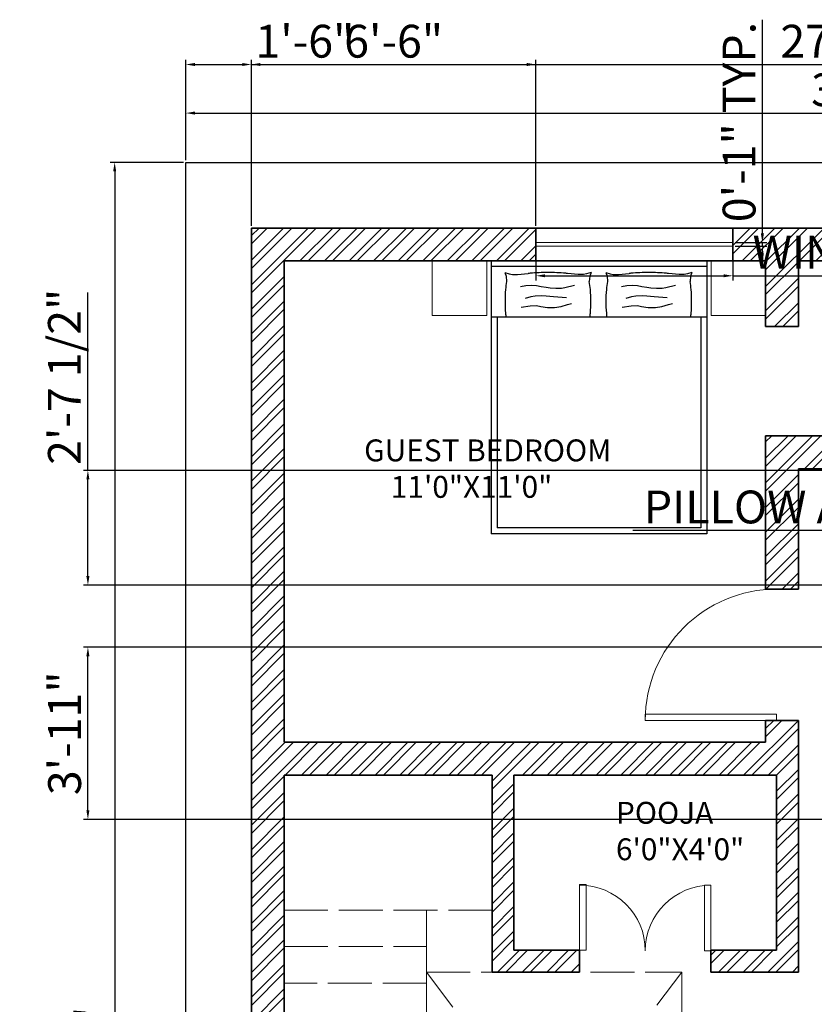
# Model space of a CAD drawing. Units: inches. Extents: x 638 to 1853, y 4393 to 5041.
# Tile 2 of 6: x 638 to 856, y 4693 to 4963. Entities that reach past the tile are written whole.
import ezdxf

# ---------------------------------------------------------------- set-up
doc = ezdxf.new("R2010")
doc.units = ezdxf.units.IN
doc.linetypes.add('ACAD_ISO02W100', pattern=[15, 12, -3])
for name, color, linetype, lineweight in [('A-ANNO-DIMS', 2, 'Continuous', 18), ('A-AREA-IDEN', 7, 'Continuous', 18), ('A-DOOR', 4, 'Continuous', 18), ('A-FLOR-STRS', 7, 'Continuous', 18), ('A-FLOR-STRS-HIDN', 7, 'ACAD_ISO02W100', 18), ('A-FURN', 26, 'Continuous', 13), ('A-GLAZ', 5, 'Continuous', 18), ('A-WALL', 7, 'Continuous', 35), ('A-WALL-PATT', 251, 'Continuous', 13), ('C-PROP', 7, 'Continuous', 25)]:
    doc.layers.add(name, color=color, linetype=linetype, lineweight=lineweight)
doc.layers.add('supurgelik', color=31, linetype='Continuous')
doc.layers.add('TASLAR', color=32, linetype='Continuous')
doc.styles.get("Standard").update_dxf_attribs({"font": 'arial.ttf'})
doc.dimstyles.new('ISO-25', dxfattribs={"dimtxt": 9, "dimasz": 2.5, "dimexe": 1.25, "dimexo": 0.625, "dimtad": 1, "dimdec": 1, "dimlunit": 3, "dimtxsty": 'Standard', "dimcen": 2.5, "dimadec": 0, "dimazin": 0, "dimtfac": 1, "dimtdec": 1, "dimtmove": 0, "dimatfit": 3, "dimfxl": 1, "dimarcsym": 0})

# ---------------------------------------------------------------- blocks, each defined once
blk = doc.blocks.new('*U4')
for p, q in [((0, 0), (0, -6)), ((36, 0), (36, -6))]:
    blk.add_line(p, q)
blk.add_lwpolyline([(0, 0), (0, 36), (1.75, 36), (1.75, 0)], close=True)
blk.add_arc((0, 0), 36, 0, 90)
blk = doc.blocks.new('hgjgh')
at = {"layer": 'supurgelik'}
for p, q in [((85993.81, -4751.89), (85843.81, -4751.89)), ((85853.26, -4756.05), (85856.29, -4757)), ((85853.26, -4756.05), (85854.18, -4758.49)), ((85854.18, -4758.49), (85854.49, -4762.19)), ((85856.29, -4757), (85858.52, -4757.5)), ((85858.52, -4757.5), (85862.12, -4757.37)), ((85862.12, -4757.37), (85869.57, -4756.72)), ((85904.4, -4757.37), (85896.95, -4756.72)), ((85908, -4757.5), (85904.4, -4757.37)), ((85910.23, -4757), (85908, -4757.5)), ((85913.26, -4756.05), (85910.23, -4757)), ((85912.34, -4758.49), (85912.03, -4762.19)), ((85913.26, -4756.05), (85912.34, -4758.49)), ((85923.48, -4756.05), (85926.51, -4757)), ((85923.48, -4756.05), (85924.4, -4758.49)), ((85924.4, -4758.49), (85924.71, -4762.19)), ((85926.51, -4757), (85928.74, -4757.5)), ((85928.74, -4757.5), (85932.34, -4757.37)), ((85932.34, -4757.37), (85939.79, -4756.72)), ((85974.62, -4757.37), (85967.17, -4756.72)), ((85978.22, -4757.5), (85974.62, -4757.37)), ((85980.45, -4757), (85978.22, -4757.5)), ((85983.48, -4756.05), (85980.45, -4757)), ((85982.56, -4758.49), (85982.25, -4762.19)), ((85983.48, -4756.05), (85982.56, -4758.49)), ((85864.23, -4765.86), (85867.95, -4764.99)), ((85867.95, -4764.99), (85871.91, -4764.87)), ((85871.91, -4764.87), (85875.39, -4765.12)), ((85875.39, -4765.12), (85878.49, -4765.74)), ((85895.1, -4766.36), (85901.8, -4764.87)), ((85934.44, -4765.86), (85938.16, -4764.99)), ((85938.16, -4764.99), (85942.13, -4764.87)), ((85942.13, -4764.87), (85945.6, -4765.12)), ((85945.6, -4765.12), (85948.7, -4765.74)), ((85965.32, -4766.36), (85972.02, -4764.87)), ((85878.86, -4772.3), (85874.27, -4772.55)), ((85878.49, -4765.74), (85881.96, -4766.23)), ((85881.96, -4772.55), (85878.86, -4772.3)), ((85881.96, -4766.23), (85884.81, -4766.61)), ((85884.81, -4766.61), (85888.65, -4766.85)), ((85888.65, -4766.85), (85892.62, -4766.85)), ((85892.62, -4766.85), (85895.1, -4766.36)), ((85949.08, -4772.3), (85944.49, -4772.55)), ((85948.7, -4765.74), (85952.18, -4766.23)), ((85952.18, -4772.55), (85949.08, -4772.3)), ((85952.18, -4766.23), (85955.03, -4766.61)), ((85955.03, -4766.61), (85958.87, -4766.85)), ((85958.87, -4766.85), (85962.84, -4766.85)), ((85962.84, -4766.85), (85965.32, -4766.36)), ((85871.29, -4773.05), (85867.33, -4774.04)), ((85870.92, -4779.28), (85875.39, -4779.03)), ((85874.27, -4772.55), (85871.29, -4773.05)), ((85875.39, -4779.03), (85878.24, -4779.65)), ((85887.04, -4773.05), (85881.96, -4772.55)), ((85890.14, -4773.3), (85887.04, -4773.05)), ((85896.09, -4773.67), (85890.14, -4773.3)), ((85892.37, -4779.65), (85896.96, -4778.41)), ((85896.96, -4778.41), (85899.69, -4777.54)), ((85941.51, -4773.05), (85937.54, -4774.04)), ((85941.14, -4779.28), (85945.6, -4779.03)), ((85944.49, -4772.55), (85941.51, -4773.05)), ((85945.6, -4779.03), (85948.46, -4779.65)), ((85957.26, -4773.05), (85952.18, -4772.55)), ((85960.36, -4773.3), (85957.26, -4773.05)), ((85966.31, -4773.67), (85960.36, -4773.3)), ((85962.59, -4779.65), (85967.18, -4778.41)), ((85967.18, -4778.41), (85969.91, -4777.54)), ((85864.72, -4780.15), (85870.92, -4779.28)), ((85878.24, -4779.65), (85882.95, -4780.4)), ((85882.95, -4780.4), (85887.91, -4780.4)), ((85887.91, -4780.4), (85892.37, -4779.65)), ((85934.94, -4780.15), (85941.14, -4779.28)), ((85948.46, -4779.65), (85953.17, -4780.4)), ((85953.17, -4780.4), (85958.13, -4780.4)), ((85958.13, -4780.4), (85962.59, -4779.65)), ((85993.81, -4787.2), (85843.81, -4787.2)), ((85847.81, -4787.2), (85847.81, -4933.89)), ((85989.81, -4787.2), (85989.81, -4933.89)), ((85989.81, -4933.89), (85847.81, -4933.89))]:
    blk.add_line(p, q, dxfattribs=at)
for centre, radius, start, end in [((85877.36, -4828.49), 72.19, 95.13619, 96.19323), ((85883.26, -4894.18), 138.14, 90, 95.13619), ((85883.26, -4894.18), 138.14, 84.86381, 90), ((85889.16, -4828.49), 72.19, 83.80677, 84.86381), ((85947.57, -4828.49), 72.19, 95.13619, 96.19323), ((85953.48, -4894.18), 138.14, 90, 95.13619), ((85953.48, -4894.18), 138.14, 84.86381, 90), ((85959.38, -4828.49), 72.19, 83.80677, 84.86381), ((85905.8, -4772.08), 52.26, 169.08956, 175.30047), ((85860.72, -4772.08), 52.26, 4.69953, 10.91044), ((85976.02, -4772.08), 52.26, 169.08956, 175.30047), ((85930.94, -4772.08), 52.26, 4.69953, 10.91044), ((85954.09, -4776.05), 100.71, 175.30047, 180), ((85812.43, -4776.05), 100.71, 0, 4.69953), ((86024.31, -4776.05), 100.71, 175.30047, 180), ((85882.65, -4776.05), 100.71, 0, 4.69953), ((85954.09, -4776.05), 100.71, 180, 184.69953), ((85812.43, -4776.05), 100.71, 355.30047, 0), ((86024.31, -4776.05), 100.71, 180, 184.69953), ((85882.65, -4776.05), 100.71, 355.30047, 0), ((85905.8, -4780.02), 52.26, 184.69953, 187.89725), ((85860.72, -4780.02), 52.26, 352.10275, 355.30047), ((85976.02, -4780.02), 52.26, 184.69953, 187.89725), ((85930.94, -4780.02), 52.26, 352.10275, 355.30047)]:
    blk.add_arc(centre, radius, start, end, dxfattribs=at)
at = {"layer": 'TASLAR'}
for p, q in [((85843.81, -4747.89), (85843.81, -4937.89)), ((85993.81, -4747.89), (85843.81, -4747.89)), ((85993.81, -4747.89), (85993.81, -4937.89)), ((85993.81, -4937.89), (85843.81, -4937.89))]:
    blk.add_line(p, q, dxfattribs=at)
blk = doc.blocks.new('*D16')
at = {"layer": 'A-ANNO-DIMS', "color": 0, "lineweight": -2, "transparency": 16777216}
for p, q in [((683.34, 4924.82), (683.34, 4938.95)), ((685.84, 4937.7), (1040.84, 4937.7)), ((1043.34, 4924.82), (1043.34, 4938.95))]:
    blk.add_line(p, q, dxfattribs=at)
at = {"layer": 'A-ANNO-DIMS', "color": 0, "transparency": 16777216}
for points in [[(685.84, 4938.12), (685.84, 4937.29), (683.34, 4937.7)], [(1040.84, 4938.12), (1040.84, 4937.29), (1043.34, 4937.7)]]:
    blk.add_solid(points, dxfattribs=at)
at = {"layer": 'Defpoints', "color": 0, "transparency": 16777216}
for p in [(1043.34, 4937.7), (683.34, 4924.19), (1043.34, 4924.19)]:
    blk.add_point(p, dxfattribs=at)
at = {"layer": 'A-ANNO-DIMS', "color": 0, "transparency": 16777216, "insert": (863.34, 4942.93), "char_height": 9, "attachment_point": 5}
blk.add_mtext("30'", dxfattribs=at)
blk = doc.blocks.new('*D17')
at = {"layer": 'A-ANNO-DIMS', "color": 0, "lineweight": -2, "transparency": 16777216}
for p, q in [((682.72, 4924.19), (662.61, 4924.19)), ((663.86, 4921.69), (663.86, 4446.69)), ((682.72, 4444.19), (662.61, 4444.19))]:
    blk.add_line(p, q, dxfattribs=at)
at = {"layer": 'A-ANNO-DIMS', "color": 0, "transparency": 16777216}
for points in [[(663.44, 4921.69), (664.28, 4921.69), (663.86, 4924.19)], [(663.44, 4446.69), (664.28, 4446.69), (663.86, 4444.19)]]:
    blk.add_solid(points, dxfattribs=at)
at = {"layer": 'Defpoints', "color": 0, "transparency": 16777216}
for p in [(683.34, 4924.19), (663.86, 4444.19), (683.34, 4444.19)]:
    blk.add_point(p, dxfattribs=at)
at = {"layer": 'A-ANNO-DIMS', "color": 0, "transparency": 16777216, "insert": (658.64, 4684.19), "char_height": 9, "attachment_point": 5, "rotation": 90}
blk.add_mtext("40'", dxfattribs=at)
blk = doc.blocks.new('BED-NIGHTSTAND-15')
blk.add_lwpolyline([(0, 14.98), (14.98, 14.98), (14.98, 0), (0, 0)], close=True)
blk = doc.blocks.new('WINDOW-GLAZING-54IN')
for p, q in [((0, 1), (54, 1)), ((0, 0), (54, 0))]:
    blk.add_line(p, q)
blk = doc.blocks.new('STAIR-WELL-OPENING')
for p, q in [((0, 93), (70, 0)), ((0, 0), (70, 93))]:
    blk.add_line(p, q)
blk.add_lwpolyline([(0, 93), (70, 93), (70, 0), (0, 0)], close=True)
blk = doc.blocks.new('*D44')
at = {"layer": 'A-ANNO-DIMS', "color": 0, "lineweight": -2, "transparency": 16777216}
for p, q in [((926.95, 4824.56), (926.95, 4822.01)), ((939.81, 4824.56), (939.81, 4822.01)), ((926.95, 4823.26), (805.91, 4823.26)), ((937.31, 4823.26), (929.45, 4823.26))]:
    blk.add_line(p, q, dxfattribs=at)
at = {"layer": 'A-ANNO-DIMS', "color": 0, "transparency": 16777216}
for points in [[(929.45, 4823.67), (929.45, 4822.84), (926.95, 4823.26)], [(937.31, 4823.67), (937.31, 4822.84), (939.81, 4823.26)]]:
    blk.add_solid(points, dxfattribs=at)
at = {"layer": 'Defpoints', "color": 0, "transparency": 16777216}
for p in [(926.95, 4825.19), (939.81, 4825.19), (926.95, 4823.26)]:
    blk.add_point(p, dxfattribs=at)
at = {"layer": 'A-ANNO-DIMS', "color": 0, "transparency": 16777216, "insert": (865.18, 4828.54), "char_height": 9, "attachment_point": 5}
blk.add_mtext('PILLOW A 1\'-1" TYP.', dxfattribs=at)
blk = doc.blocks.new('*D46')
at = {"layer": 'A-ANNO-DIMS', "color": 0, "lineweight": -2, "transparency": 16777216}
for p, q in [((779.34, 4900.57), (779.34, 4891.84)), ((833.34, 4900.57), (833.34, 4891.84)), ((781.84, 4893.09), (830.84, 4893.09)), ((833.34, 4893.09), (950.98, 4893.09))]:
    blk.add_line(p, q, dxfattribs=at)
at = {"layer": 'A-ANNO-DIMS', "color": 0, "transparency": 16777216}
for points in [[(781.84, 4893.51), (781.84, 4892.68), (779.34, 4893.09)], [(830.84, 4893.51), (830.84, 4892.68), (833.34, 4893.09)]]:
    blk.add_solid(points, dxfattribs=at)
at = {"layer": 'Defpoints', "color": 0, "transparency": 16777216}
for p in [(779.34, 4901.19), (833.34, 4901.19), (833.34, 4893.09)]:
    blk.add_point(p, dxfattribs=at)
at = {"layer": 'A-ANNO-DIMS', "color": 0, "transparency": 16777216, "insert": (893.41, 4898.38), "char_height": 9, "attachment_point": 5}
blk.add_mtext('WINDOW 4\'-6" TYP.', dxfattribs=at)
blk = doc.blocks.new('*D47')
at = {"layer": 'A-ANNO-DIMS', "color": 0, "lineweight": -2, "transparency": 16777216}
for p, q in [((841.44, 4904.69), (841.44, 4963.3)), ((833.97, 4902.19), (842.69, 4902.19)), ((833.97, 4901.19), (842.69, 4901.19)), ((841.44, 4901.19), (841.44, 4902.19)), ((841.44, 4898.69), (841.44, 4896.19))]:
    blk.add_line(p, q, dxfattribs=at)
at = {"layer": 'A-ANNO-DIMS', "color": 0, "transparency": 16777216}
for points in [[(841.02, 4904.69), (841.86, 4904.69), (841.44, 4902.19)], [(841.02, 4898.69), (841.86, 4898.69), (841.44, 4901.19)]]:
    blk.add_solid(points, dxfattribs=at)
at = {"layer": 'Defpoints', "color": 0, "transparency": 16777216}
for p in [(833.34, 4902.19), (833.34, 4901.19), (841.44, 4902.19)]:
    blk.add_point(p, dxfattribs=at)
at = {"layer": 'A-ANNO-DIMS', "color": 0, "transparency": 16777216, "insert": (836.22, 4935.25), "char_height": 9, "attachment_point": 5, "rotation": 90}
blk.add_mtext('0\'-1" TYP.', dxfattribs=at)
blk = doc.blocks.new('*D62')
at = {"layer": 'A-ANNO-DIMS', "color": 0, "lineweight": -2, "transparency": 16777216}
for p, q in [((786.73, 4678.11), (786.73, 4689.96)), ((861.6, 4678.11), (861.6, 4689.96)), ((789.23, 4688.71), (859.1, 4688.71)), ((861.6, 4688.71), (964.27, 4688.71))]:
    blk.add_line(p, q, dxfattribs=at)
at = {"layer": 'A-ANNO-DIMS', "color": 0, "transparency": 16777216}
for points in [[(789.23, 4689.13), (789.23, 4688.3), (786.73, 4688.71)], [(859.1, 4689.13), (859.1, 4688.3), (861.6, 4688.71)]]:
    blk.add_solid(points, dxfattribs=at)
at = {"layer": 'Defpoints', "color": 0, "transparency": 16777216}
for p in [(861.6, 4688.71), (786.73, 4677.48), (861.6, 4677.48)]:
    blk.add_point(p, dxfattribs=at)
at = {"layer": 'A-ANNO-DIMS', "color": 0, "transparency": 16777216, "insert": (914.18, 4694), "char_height": 9, "attachment_point": 5}
blk.add_mtext('DINING SET 6\'-3"', dxfattribs=at)
blk = doc.blocks.new('*D74')
at = {"layer": 'A-ANNO-DIMS', "color": 0, "lineweight": -2, "transparency": 16777216}
for p, q in [((701.34, 4906.82), (701.34, 4952.27)), ((703.84, 4951.02), (1022.84, 4951.02)), ((1025.34, 4906.82), (1025.34, 4952.27))]:
    blk.add_line(p, q, dxfattribs=at)
at = {"layer": 'A-ANNO-DIMS', "color": 0, "transparency": 16777216}
for points in [[(703.84, 4951.44), (703.84, 4950.6), (701.34, 4951.02)], [(1022.84, 4951.44), (1022.84, 4950.6), (1025.34, 4951.02)]]:
    blk.add_solid(points, dxfattribs=at)
at = {"layer": 'Defpoints', "color": 0, "transparency": 16777216}
for p in [(1025.34, 4951.02), (701.34, 4906.19), (1025.34, 4906.19)]:
    blk.add_point(p, dxfattribs=at)
at = {"layer": 'A-ANNO-DIMS', "color": 0, "transparency": 16777216, "insert": (863.34, 4956.24), "char_height": 9, "attachment_point": 5}
blk.add_mtext('27\'-0"', dxfattribs=at)
blk = doc.blocks.new('*D76')
at = {"layer": 'A-ANNO-DIMS', "color": 0, "lineweight": -2, "transparency": 16777216}
for p, q in [((683.34, 4924.82), (683.34, 4952.27)), ((685.84, 4951.02), (698.84, 4951.02)), ((701.34, 4906.82), (701.34, 4952.27)), ((701.34, 4951.02), (728.17, 4951.02))]:
    blk.add_line(p, q, dxfattribs=at)
at = {"layer": 'A-ANNO-DIMS', "color": 0, "transparency": 16777216}
for points in [[(685.84, 4951.44), (685.84, 4950.6), (683.34, 4951.02)], [(698.84, 4951.44), (698.84, 4950.6), (701.34, 4951.02)]]:
    blk.add_solid(points, dxfattribs=at)
at = {"layer": 'Defpoints', "color": 0, "transparency": 16777216}
for p in [(701.34, 4951.02), (683.34, 4924.19), (701.34, 4906.19)]:
    blk.add_point(p, dxfattribs=at)
at = {"layer": 'A-ANNO-DIMS', "color": 0, "transparency": 16777216, "insert": (716, 4956.24), "char_height": 9, "attachment_point": 5}
blk.add_mtext('1\'-6"', dxfattribs=at)
blk = doc.blocks.new('*D80')
at = {"layer": 'A-ANNO-DIMS', "color": 0, "lineweight": -2, "transparency": 16777216}
for p, q in [((701.34, 4906.82), (701.34, 4952.27)), ((703.84, 4951.02), (776.84, 4951.02)), ((779.34, 4906.82), (779.34, 4952.27))]:
    blk.add_line(p, q, dxfattribs=at)
at = {"layer": 'A-ANNO-DIMS', "color": 0, "transparency": 16777216}
for points in [[(703.84, 4951.44), (703.84, 4950.6), (701.34, 4951.02)], [(776.84, 4951.44), (776.84, 4950.6), (779.34, 4951.02)]]:
    blk.add_solid(points, dxfattribs=at)
at = {"layer": 'Defpoints', "color": 0, "transparency": 16777216}
for p in [(779.34, 4951.02), (701.34, 4906.19), (779.34, 4906.19)]:
    blk.add_point(p, dxfattribs=at)
at = {"layer": 'A-ANNO-DIMS', "color": 0, "transparency": 16777216, "insert": (740.34, 4956.24), "char_height": 9, "attachment_point": 5}
blk.add_mtext('6\'-6"', dxfattribs=at)
blk = doc.blocks.new('*D85')
at = {"layer": 'A-ANNO-DIMS', "color": 0, "lineweight": -2, "transparency": 16777216}
for p, q in [((939.25, 4791.29), (655.27, 4791.29)), ((656.52, 4746.54), (656.52, 4788.79)), ((939.25, 4744.04), (655.27, 4744.04))]:
    blk.add_line(p, q, dxfattribs=at)
at = {"layer": 'A-ANNO-DIMS', "color": 0, "transparency": 16777216}
for points in [[(656.1, 4788.79), (656.93, 4788.79), (656.52, 4791.29)], [(656.1, 4746.54), (656.93, 4746.54), (656.52, 4744.04)]]:
    blk.add_solid(points, dxfattribs=at)
at = {"layer": 'Defpoints', "color": 0, "transparency": 16777216}
for p in [(656.52, 4791.29), (939.87, 4791.29), (939.87, 4744.04)]:
    blk.add_point(p, dxfattribs=at)
at = {"layer": 'A-ANNO-DIMS', "color": 0, "transparency": 16777216, "insert": (651.29, 4767.66), "char_height": 9, "attachment_point": 5, "rotation": 90}
blk.add_mtext('3\'-11"', dxfattribs=at)
blk = doc.blocks.new('*D87')
at = {"layer": 'A-ANNO-DIMS', "color": 0, "lineweight": -2, "transparency": 16777216}
for p, q in [((656.52, 4839.74), (656.52, 4888.54)), ((892.19, 4839.74), (655.27, 4839.74)), ((656.52, 4810.75), (656.52, 4837.24)), ((892.19, 4808.25), (655.27, 4808.25))]:
    blk.add_line(p, q, dxfattribs=at)
at = {"layer": 'A-ANNO-DIMS', "color": 0, "transparency": 16777216}
for points in [[(656.1, 4837.24), (656.93, 4837.24), (656.52, 4839.74)], [(656.1, 4810.75), (656.93, 4810.75), (656.52, 4808.25)]]:
    blk.add_solid(points, dxfattribs=at)
at = {"layer": 'Defpoints', "color": 0, "transparency": 16777216}
for p in [(656.52, 4839.74), (892.82, 4839.74), (892.82, 4808.25)]:
    blk.add_point(p, dxfattribs=at)
at = {"layer": 'A-ANNO-DIMS', "color": 0, "transparency": 16777216, "insert": (651.24, 4865.39), "char_height": 9, "attachment_point": 5, "rotation": 90}
blk.add_mtext('2\'-7 1/2"', dxfattribs=at)

msp = doc.modelspace()

# ---------------------------------------------------------------- hatches: boundary and pattern name
at = {"layer": 'A-WALL-PATT', "transparency": 33554687}
h = msp.add_hatch(dxfattribs=at)
h.set_pattern_fill('ANSI32', color=256, scale=0.5)
h.paths.add_polyline_path([(779.34, 4906.19), (701.34, 4906.19), (701.34, 4531.19), (710.34, 4531.19), (710.34, 4561.19), (758.34, 4561.19), (758.34, 4528.19), (764.34, 4528.19), (767.34, 4528.19), (767.34, 4561.19), (821.34, 4561.19), (821.34, 4570.19), (710.34, 4570.19), (710.34, 4756.19), (767.34, 4756.19), (767.34, 4702.19), (791.34, 4702.19), (791.34, 4708.19), (773.34, 4708.19), (773.34, 4756.19), (845.34, 4756.19), (845.34, 4708.19), (827.35, 4708.19), (827.35, 4705.02), (827.34, 4702.19), (851.34, 4702.19), (851.34, 4771.19), (845.34, 4771.19), (842.34, 4771.19), (842.34, 4765.19), (710.34, 4765.19), (710.34, 4897.19), (779.34, 4897.19)])
h.paths.add_polyline_path([(1025.34, 4906.19), (833.34, 4906.19), (833.34, 4897.19), (842.34, 4897.19), (842.34, 4882.21), (842.34, 4879.19), (851.34, 4879.19), (851.34, 4897.19), (914.34, 4897.19), (914.34, 4879.19), (920.34, 4879.19), (920.34, 4897.19), (1016.34, 4897.19), (1016.34, 4885.19), (1025.34, 4885.19)])
h.paths.add_polyline_path([(851.34, 4840.19), (1016.34, 4840.19), (1016.34, 4780.19), (1025.34, 4780.19), (1025.34, 4861.19), (1016.34, 4861.19), (1016.34, 4849.19), (842.34, 4849.19), (842.34, 4807.19), (851.34, 4807.19)])
h.paths.add_polyline_path([(1025.34, 4708.19), (1016.34, 4708.19), (1016.34, 4694.92), (1016.34, 4648.19), (996.84, 4648.19), (996.84, 4639.19), (1025.34, 4639.19)])
h.paths.add_polyline_path([(972.84, 4648.19), (944.34, 4648.19), (944.34, 4561.19), (953.34, 4561.19), (953.34, 4639.19), (972.84, 4639.19)])
h.paths.add_polyline_path([(896.34, 4648.19), (887.34, 4648.19), (887.34, 4570.19), (863.34, 4570.19), (863.34, 4561.19), (887.34, 4561.19), (887.34, 4552.19), (896.34, 4552.19), (896.34, 4561.19), (904.34, 4561.19), (904.34, 4567.19), (904.34, 4570.19), (896.34, 4570.19)])
h.paths.add_polyline_path([(896.34, 4504.19), (887.34, 4504.19), (887.34, 4465.19), (839.34, 4465.19), (839.34, 4456.19), (896.34, 4456.19)])
h.paths.add_polyline_path([(779.34, 4465.19), (767.34, 4465.19), (767.34, 4498.19), (758.34, 4498.19), (758.34, 4465.19), (710.34, 4465.19), (710.34, 4495.19), (701.34, 4495.19), (701.34, 4456.19), (779.34, 4456.19)])
h.paths.add_polyline_path([(865.86, 4868.68), (912.64, 4868.68), (912.64, 4891.07), (865.86, 4891.07)], flags=9)
h.paths.add_polyline_path([(730.31, 4828.82), (807.82, 4828.82), (807.82, 4851.21), (730.31, 4851.21)], flags=25)

# ---------------------------------------------------------------- linework, layer by layer
at = {"layer": 'A-DOOR'}
for p, q in [((791.34, 4708.19), (791.34, 4705.19)), ((827.35, 4708.02), (827.35, 4705.02))]:
    msp.add_line(p, q, dxfattribs=at)
for points in [[(791.34, 4708.19), (791.34, 4726.19), (793.09, 4726.19), (793.09, 4708.19)], [(827.35, 4708.02), (827.35, 4726.02), (825.6, 4726.02), (825.6, 4708.02)]]:
    msp.add_lwpolyline(points, close=True, dxfattribs=at)
for centre, start, end in [((791.35, 4708.02), 0, 90), ((827.35, 4708.02), 90, 180)]:
    msp.add_arc(centre, 18, start, end, dxfattribs=at)
at = {"layer": 'A-FLOR-STRS'}
msp.add_line((749.34, 4570.19), (749.34, 4719.19), dxfattribs=at)
at = {"layer": 'A-FLOR-STRS-HIDN'}
for p, q in [((767.34, 4719.19), (710.34, 4719.19)), ((710.34, 4709.19), (749.34, 4709.19)), ((749.34, 4699.19), (710.34, 4699.19))]:
    msp.add_line(p, q, dxfattribs=at)
at = {"layer": 'A-FURN'}
msp.add_lwpolyline([(827.36, 4897.19), (842.34, 4897.19), (842.34, 4882.21), (827.36, 4882.21)], close=True, dxfattribs=at)
at = {"layer": 'A-WALL'}
for p, q in [((701.34, 4906.19), (1025.34, 4906.19)), ((701.34, 4456.19), (701.34, 4906.19)), ((779.34, 4897.19), (779.34, 4906.19)), ((833.34, 4897.19), (833.34, 4906.19)), ((710.34, 4897.19), (842.34, 4897.19)), ((710.34, 4765.19), (710.34, 4897.19)), ((842.34, 4879.19), (842.34, 4897.19)), ((851.34, 4897.19), (914.34, 4897.19)), ((851.34, 4879.19), (851.34, 4897.19)), ((842.34, 4879.19), (851.34, 4879.19)), ((842.34, 4849.19), (1016.34, 4849.19)), ((842.34, 4807.19), (842.34, 4849.19)), ((851.34, 4840.19), (1016.34, 4840.19)), ((851.34, 4807.19), (851.34, 4840.19)), ((842.34, 4807.19), (851.34, 4807.19)), ((842.34, 4771.19), (851.34, 4771.19)), ((842.34, 4765.19), (842.34, 4771.19)), ((851.34, 4702.19), (851.34, 4771.19)), ((710.34, 4765.19), (842.34, 4765.19)), ((710.34, 4756.19), (767.34, 4756.19)), ((710.34, 4570.19), (710.34, 4756.19)), ((767.34, 4702.19), (767.34, 4756.19)), ((773.34, 4756.19), (845.34, 4756.19)), ((773.34, 4708.19), (773.34, 4756.19)), ((845.34, 4708.19), (845.34, 4756.19)), ((773.34, 4708.19), (791.34, 4708.19)), ((791.34, 4708.19), (791.34, 4702.19)), ((827.34, 4708.19), (845.34, 4708.19)), ((827.34, 4708.19), (827.34, 4702.19)), ((767.34, 4702.19), (791.34, 4702.19)), ((827.34, 4702.19), (851.34, 4702.19))]:
    msp.add_line(p, q, dxfattribs=at)
at = {"layer": 'C-PROP'}
msp.add_lwpolyline([(683.34, 4924.19), (1043.34, 4924.19), (1043.34, 4444.19), (683.34, 4444.19)], close=True, dxfattribs=at)

# ---------------------------------------------------------------- block references
at = {"layer": 'A-DOOR', "rotation": 90}
msp.add_blockref('*U4', (845.34, 4771.19), dxfattribs=at)
at = {"layer": 'A-FLOR-STRS-HIDN'}
msp.add_blockref('STAIR-WELL-OPENING', (749.34, 4609.19), dxfattribs=at)
at = {"layer": 'A-FURN'}
msp.add_blockref('BED-NIGHTSTAND-15', (750.95, 4882.21), dxfattribs=at)
at = {"layer": 'A-FURN', "xscale": 0.393701, "yscale": 0.393701, "zscale": 0.393701}
msp.add_blockref('hgjgh', (-33029.68, 6766.44), dxfattribs=at)
at = {"layer": 'A-GLAZ'}
msp.add_blockref('WINDOW-GLAZING-54IN', (779.34, 4901.19), dxfattribs=at)

# ---------------------------------------------------------------- texts
at = {"layer": 'A-AREA-IDEN', "char_height": 6, "attachment_point": 1}
for s, insert in [('GUEST BEDROOM\\P    11\'0"X11\'0"', (732.25, 4848.22)), ('POOJA\\P6\'0"X4\'0"', (801.3, 4748.86))]:
    msp.add_mtext_dynamic_manual_height_columns(s, width=77.4832, gutter_width=12.5, heights=[0], dxfattribs=dict(at, insert=insert))

# ---------------------------------------------------------------- dimensions: what is measured, and where the dimension line sits
at = {"layer": 'A-ANNO-DIMS'}
for base, p1, p2, override, picture, middle in [((701.34, 4951.02), (683.34, 4924.19), (701.34, 4906.19), {"dimdec": 1, "dimlfac": 1, "dimrnd": 0, "dimzin": 1, "dimdsep": 46, "dimlunit": 4, "dimfrac": 2}, '*D76', (716, 4956.24)), ((1025.34, 4951.02), (701.34, 4906.19), (1025.34, 4906.19), {"dimdec": 1, "dimlfac": 1, "dimrnd": 0, "dimzin": 1, "dimdsep": 46, "dimlunit": 4, "dimfrac": 2}, '*D74', (863.34, 4956.24)), ((779.34, 4951.02), (701.34, 4906.19), (779.34, 4906.19), {"dimdec": 1, "dimlfac": 1, "dimrnd": 0, "dimzin": 1, "dimdsep": 46, "dimlunit": 4, "dimfrac": 2}, '*D80', (740.34, 4956.24)), ((1043.34, 4937.7), (683.34, 4924.19), (1043.34, 4924.19), {"dimclrd": 0, "dimclre": 0, "dimclrt": 0}, '*D16', (863.34, 4942.93))]:
    dim = msp.add_linear_dim(base=base, p1=p1, p2=p2, dimstyle='ISO-25', override=override, dxfattribs=at)
    dim.commit()
    dim.dimension.update_dxf_attribs({"geometry": picture, "text_midpoint": middle})
for base, p1, p2, angle, text, picture, middle in [((841.44, 4902.19), (833.34, 4901.19), (833.34, 4902.19), 90, '<> TYP.', '*D47', (836.22, 4935.25)), ((926.95, 4823.26), (939.81, 4825.19), (926.95, 4825.19), 180, 'PILLOW A <> TYP.', '*D44', (865.18, 4828.54))]:
    dim = msp.add_linear_dim(base=base, p1=p1, p2=p2, angle=angle, text=text, dimstyle='ISO-25', override={"dimdec": 1, "dimlfac": 1, "dimrnd": 0, "dimzin": 1, "dimdsep": 46, "dimlunit": 4, "dimfrac": 2}, dxfattribs=at)
    dim.commit()
    dim.dimension.update_dxf_attribs({"geometry": picture, "text_midpoint": middle})
for base, p1, p2, override, picture, middle in [((663.86, 4444.19), (683.34, 4924.19), (683.34, 4444.19), {"dimclrd": 0, "dimclre": 0, "dimclrt": 0}, '*D17', (658.64, 4684.19)), ((656.52, 4839.74), (892.82, 4808.25), (892.82, 4839.74), {"dimdec": 1, "dimlfac": 1, "dimrnd": 0, "dimzin": 1, "dimdsep": 46, "dimlunit": 4, "dimfrac": 2}, '*D87', (651.24, 4865.39)), ((656.5159, 4791.2857), (939.8728, 4744.0416), (939.8728, 4791.2857), {"dimdec": 1, "dimlfac": 1, "dimrnd": 0, "dimzin": 1, "dimdsep": 46, "dimlunit": 4, "dimfrac": 2}, '*D85', (651.2927, 4767.6637))]:
    dim = msp.add_linear_dim(base=base, p1=p1, p2=p2, angle=90, dimstyle='ISO-25', override=override, dxfattribs=at)
    dim.commit()
    dim.dimension.update_dxf_attribs({"geometry": picture, "text_midpoint": middle})
for base, p1, p2, text, picture, middle in [((833.34, 4893.09), (779.34, 4901.19), (833.34, 4901.19), 'WINDOW <> TYP.', '*D46', (893.41, 4898.38)), ((861.6, 4688.71), (786.73, 4677.48), (861.6, 4677.48), 'DINING SET <>', '*D62', (914.18, 4694))]:
    dim = msp.add_linear_dim(base=base, p1=p1, p2=p2, text=text, dimstyle='ISO-25', override={"dimdec": 1, "dimlfac": 1, "dimrnd": 0, "dimzin": 1, "dimdsep": 46, "dimlunit": 4, "dimfrac": 2}, dxfattribs=at)
    dim.commit()
    dim.dimension.update_dxf_attribs({"geometry": picture, "text_midpoint": middle})

doc.saveas('drawing.dxf')
